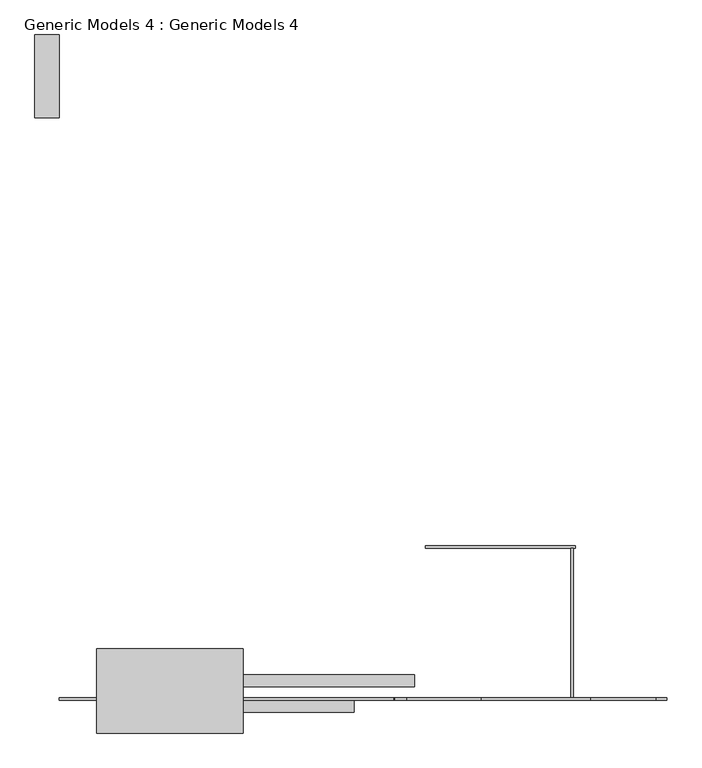
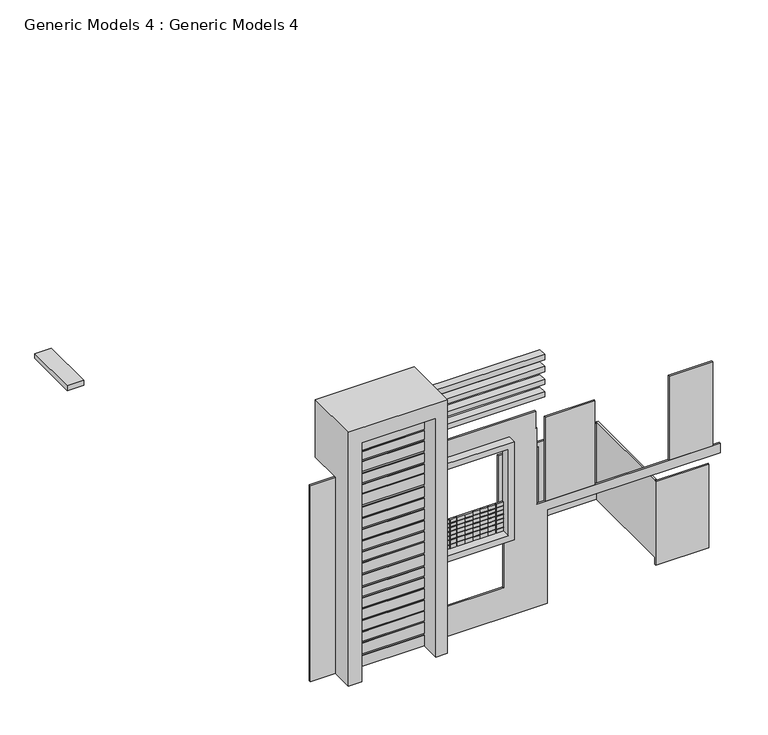
"""IFC4 building model written with IfcOpenShell, lengths in millimetres: proxy geometry, Generic Models 4 : Generic Models 4."""

from ifc_helpers import new_model, si_unit, frame, origin, origin_with_axes, place, context, project, spatial, polyline, outline, extrude, faceted_brep, source, transform, mapped, element, save


def generic_models_4_generic_models_4_67bf9aa9(model_context):
    return source(origin(), model_context, "Body", "SolidModel", [
        extrude(outline(polyline([(-19874.3127664, -11976.0511954), (-19874.3127664, -11725.3336873), (-16074.1386697, -11725.3336873), (-16074.1386697, -11976.0511954), (-19874.3127664, -11976.0511954)])), frame((0.0, 0.0, 7756.9299202), z_axis=(0.0, 0.0, 1.0), x_axis=(1.0, 0.0, 0.0)), (0.0, 0.0, 1.0), 173.7908579),
        extrude(outline(polyline([(-19874.3127664, -11976.0511954), (-19874.3127664, -11725.3336873), (-16074.1386697, -11725.3336873), (-16074.1386697, -11976.0511954), (-19874.3127664, -11976.0511954)])), frame((0.0, 0.0, 7363.4945903), z_axis=(0.0, 0.0, 1.0), x_axis=(1.0, 0.0, 0.0)), (0.0, 0.0, 1.0), 172.4010314),
        extrude(outline(polyline([(-19874.3127664, -11976.0511954), (-19874.3127664, -11725.3336873), (-16074.1386697, -11725.3336873), (-16074.1386697, -11976.0511954), (-19874.3127664, -11976.0511954)])), frame((0.0, 0.0, 6958.2524278), z_axis=(0.0, 0.0, 1.0), x_axis=(1.0, 0.0, 0.0)), (0.0, 0.0, 1.0), 155.6173334),
        extrude(outline(polyline([(-19874.3127664, -11976.0511954), (-19874.3127664, -11725.3336873), (-16074.1386697, -11725.3336873), (-16074.1386697, -11976.0511954), (-19874.3127664, -11976.0511954)])), frame((0.0, 0.0, 6536.8664584), z_axis=(0.0, 0.0, 1.0), x_axis=(1.0, 0.0, 0.0)), (0.0, 0.0, 1.0), 161.3441341),
        extrude(outline(polyline([(-23975.6647706, 1587.5488046), (-23465.5386697, 1587.5488046), (-23465.5386697, -136.4761954), (-23975.6647706, -136.4761954), (-23975.6647706, 1587.5488046)])), frame((0.0, 0.0, 2332.8596388), z_axis=(0.0, 0.0, 1.0), x_axis=(1.0, 0.0, 0.0)), (0.0, 0.0, 1.0), 152.4),
        faceted_brep([(-19636.4886697, -12255.4511954, 3784.7260489), (-19636.4886697, -12255.4511954, 3671.2049424), (-19413.4515656, -12255.4511954, 3671.2049424), (-19413.4515656, -12255.4511954, 3784.7260489), (-19636.4886697, -12255.4511954, 3649.7991228), (-19636.4886697, -12255.4511954, 3542.7700248), (-19413.4515656, -12255.4511954, 3542.7700248), (-19413.4515656, -12255.4511954, 3649.7991228), (-19636.4886697, -12255.4511954, 3518.306231), (-19636.4886697, -12255.4511954, 3408.2191587), (-19413.4515656, -12255.4511954, 3408.2191587), (-19413.4515656, -12255.4511954, 3518.306231), (-19636.4886697, -12255.4511954, 3383.7553649), (-19636.4886697, -12255.4511954, 3271.5066224), (-19413.4515656, -12255.4511954, 3271.5066224), (-19413.4515656, -12255.4511954, 3383.7553649), (-19636.4886697, -12255.4511954, 3255.3204473), (-19636.4886697, -12255.4511954, 3137.364874), (-19413.4515656, -12255.4511954, 3137.364874), (-19413.4515656, -12255.4511954, 3255.3204473), (-19636.4886697, -12255.4511954, 2960.0023687), (-19636.4886697, -12255.4511954, 2833.3789545), (-19413.4515656, -12255.4511954, 2833.3789545), (-19413.4515656, -12255.4511954, 2960.0023687), (-19636.4886697, -12255.4511954, 3112.9010801), (-19636.4886697, -12255.4511954, 2978.3502141), (-19413.4515656, -12255.4511954, 2978.3502141), (-19413.4515656, -12255.4511954, 3112.9010801), (-17502.8886697, -12255.4511954, 3671.2049424), (-17502.8886697, -12255.4511954, 3784.7260489), (-17737.0072187, -12255.4511954, 3784.7260489), (-17737.0072187, -12255.4511954, 3671.2049424), (-17502.8886697, -12255.4511954, 3542.7700248), (-17502.8886697, -12255.4511954, 3649.7991228), (-17737.0072187, -12255.4511954, 3649.7991228), (-17737.0072187, -12255.4511954, 3542.7700248), (-17502.8886697, -12255.4511954, 3408.2191587), (-17502.8886697, -12255.4511954, 3518.306231), (-17737.0072187, -12255.4511954, 3518.306231), (-17737.0072187, -12255.4511954, 3408.2191587), (-17502.8886697, -12255.4511954, 3271.5066224), (-17502.8886697, -12255.4511954, 3383.7553649), (-17737.0072187, -12255.4511954, 3383.7553649), (-17737.0072187, -12255.4511954, 3271.5066224), (-17502.8886697, -12255.4511954, 3137.364874), (-17502.8886697, -12255.4511954, 3255.3204473), (-17737.0072187, -12255.4511954, 3255.3204473), (-17737.0072187, -12255.4511954, 3137.364874), (-17502.8886697, -12255.4511954, 2833.3789545), (-17502.8886697, -12255.4511954, 2960.0023687), (-17737.0072187, -12255.4511954, 2960.0023687), (-17737.0072187, -12255.4511954, 2833.3789545), (-17502.8886697, -12255.4511954, 2978.3502141), (-17502.8886697, -12255.4511954, 3112.9010801), (-17737.0072187, -12255.4511954, 3112.9010801), (-17737.0072187, -12255.4511954, 2978.3502141), (-19182.4143994, -12255.4511954, 3784.7260489), (-19387.1657173, -12255.4511954, 3784.7260489), (-19387.1657173, -12255.4511954, 3671.2049424), (-19182.4143994, -12255.4511954, 3671.2049424), (-18957.0386697, -12255.4511954, 3784.7260489), (-19153.1642111, -12255.4511954, 3784.7260489), (-19153.1642111, -12255.4511954, 3671.2049424), (-18957.0386697, -12255.4511954, 3671.2049424), (-18703.0386697, -12255.4511954, 3784.7260489), (-18927.140029, -12255.4511954, 3784.7260489), (-18927.140029, -12255.4511954, 3671.2049424), (-18703.0386697, -12255.4511954, 3671.2049424), (-18461.2038197, -12255.4511954, 3784.7260489), (-18685.5210952, -12255.4511954, 3784.7260489), (-18685.5210952, -12255.4511954, 3671.2049424), (-18461.2038197, -12255.4511954, 3671.2049424), (-18245.8386697, -12255.4511954, 3784.7260489), (-18433.5803118, -12255.4511954, 3784.7260489), (-18433.5803118, -12255.4511954, 3671.2049424), (-18245.8386697, -12255.4511954, 3671.2049424), (-17998.1886697, -12255.4511954, 3784.7260489), (-18218.7706288, -12255.4511954, 3784.7260489), (-18218.7706288, -12255.4511954, 3671.2049424), (-17998.1886697, -12255.4511954, 3671.2049424), (-17756.5762606, -12255.4511954, 3784.7260489), (-17975.8395726, -12255.4511954, 3784.7260489), (-17975.8395726, -12255.4511954, 3671.2049424), (-17756.5762606, -12255.4511954, 3671.2049424), (-19387.1657173, -12255.4511954, 2833.3789545), (-19182.4143994, -12255.4511954, 2833.3789545), (-19182.4143994, -12255.4511954, 2960.0023687), (-19387.1657173, -12255.4511954, 2960.0023687), (-19153.1642111, -12255.4511954, 2833.3789545), (-18957.0386697, -12255.4511954, 2833.3789545), (-18957.0386697, -12255.4511954, 2960.0023687), (-19153.1642111, -12255.4511954, 2960.0023687), (-18927.140029, -12255.4511954, 2833.3789545), (-18703.0386697, -12255.4511954, 2833.3789545), (-18703.0386697, -12255.4511954, 2960.0023687), (-18927.140029, -12255.4511954, 2960.0023687), (-18685.5210952, -12255.4511954, 2833.3789545), (-18461.2038197, -12255.4511954, 2833.3789545), (-18461.2038197, -12255.4511954, 2960.0023687), (-18685.5210952, -12255.4511954, 2960.0023687), (-18433.5803118, -12255.4511954, 2833.3789545), (-18245.8386697, -12255.4511954, 2833.3789545), (-18245.8386697, -12255.4511954, 2960.0023687), (-18433.5803118, -12255.4511954, 2960.0023687), (-18218.7706288, -12255.4511954, 2833.3789545), (-17998.1886697, -12255.4511954, 2833.3789545), (-17998.1886697, -12255.4511954, 2960.0023687), (-18218.7706288, -12255.4511954, 2960.0023687), (-17975.8395726, -12255.4511954, 2833.3789545), (-17756.5762606, -12255.4511954, 2833.3789545), (-17756.5762606, -12255.4511954, 2960.0023687), (-17975.8395726, -12255.4511954, 2960.0023687), (-19387.1657173, -12255.4511954, 3542.7700248), (-19182.4143994, -12255.4511954, 3542.7700248), (-19182.4143994, -12255.4511954, 3649.7991228), (-19387.1657173, -12255.4511954, 3649.7991228), (-19153.1642111, -12255.4511954, 3542.7700248), (-18957.0386697, -12255.4511954, 3542.7700248), (-18957.0386697, -12255.4511954, 3649.7991228), (-19153.1642111, -12255.4511954, 3649.7991228), (-18927.140029, -12255.4511954, 3542.7700248), (-18703.0386697, -12255.4511954, 3542.7700248), (-18703.0386697, -12255.4511954, 3649.7991228), (-18927.140029, -12255.4511954, 3649.7991228), (-18685.5210952, -12255.4511954, 3542.7700248), (-18461.2038197, -12255.4511954, 3542.7700248), (-18461.2038197, -12255.4511954, 3649.7991228), (-18685.5210952, -12255.4511954, 3649.7991228), (-18433.5803118, -12255.4511954, 3542.7700248), (-18245.8386697, -12255.4511954, 3542.7700248), (-18245.8386697, -12255.4511954, 3649.7991228), (-18433.5803118, -12255.4511954, 3649.7991228), (-18218.7706288, -12255.4511954, 3542.7700248), (-17998.1886697, -12255.4511954, 3542.7700248), (-17998.1886697, -12255.4511954, 3649.7991228), (-18218.7706288, -12255.4511954, 3649.7991228), (-17975.8395726, -12255.4511954, 3542.7700248), (-17756.5762606, -12255.4511954, 3542.7700248), (-17756.5762606, -12255.4511954, 3649.7991228), (-17975.8395726, -12255.4511954, 3649.7991228), (-19387.1657173, -12255.4511954, 3408.2191587), (-19182.4143994, -12255.4511954, 3408.2191587), (-19182.4143994, -12255.4511954, 3518.306231), (-19387.1657173, -12255.4511954, 3518.306231), (-19153.1642111, -12255.4511954, 3408.2191587), (-18957.0386697, -12255.4511954, 3408.2191587), (-18957.0386697, -12255.4511954, 3518.306231), (-19153.1642111, -12255.4511954, 3518.306231), (-18927.140029, -12255.4511954, 3408.2191587), (-18703.0386697, -12255.4511954, 3408.2191587), (-18703.0386697, -12255.4511954, 3518.306231), (-18927.140029, -12255.4511954, 3518.306231), (-18685.5210952, -12255.4511954, 3408.2191587), (-18461.2038197, -12255.4511954, 3408.2191587), (-18461.2038197, -12255.4511954, 3518.306231), (-18685.5210952, -12255.4511954, 3518.306231), (-18433.5803118, -12255.4511954, 3408.2191587), (-18245.8386697, -12255.4511954, 3408.2191587), (-18245.8386697, -12255.4511954, 3518.306231), (-18433.5803118, -12255.4511954, 3518.306231), (-18218.7706288, -12255.4511954, 3408.2191587), (-17998.1886697, -12255.4511954, 3408.2191587), (-17998.1886697, -12255.4511954, 3518.306231), (-18218.7706288, -12255.4511954, 3518.306231), (-17975.8395726, -12255.4511954, 3408.2191587), (-17756.5762606, -12255.4511954, 3408.2191587), (-17756.5762606, -12255.4511954, 3518.306231), (-17975.8395726, -12255.4511954, 3518.306231), (-19387.1657173, -12255.4511954, 3271.5066224), (-19182.4143994, -12255.4511954, 3271.5066224), (-19182.4143994, -12255.4511954, 3383.7553649), (-19387.1657173, -12255.4511954, 3383.7553649), (-19153.1642111, -12255.4511954, 3271.5066224), (-18957.0386697, -12255.4511954, 3271.5066224), (-18957.0386697, -12255.4511954, 3383.7553649), (-19153.1642111, -12255.4511954, 3383.7553649), (-18927.140029, -12255.4511954, 3271.5066224), (-18703.0386697, -12255.4511954, 3271.5066224), (-18703.0386697, -12255.4511954, 3383.7553649), (-18927.140029, -12255.4511954, 3383.7553649), (-18685.5210952, -12255.4511954, 3271.5066224), (-18461.2038197, -12255.4511954, 3271.5066224), (-18461.2038197, -12255.4511954, 3383.7553649), (-18685.5210952, -12255.4511954, 3383.7553649), (-18433.5803118, -12255.4511954, 3271.5066224), (-18245.8386697, -12255.4511954, 3271.5066224), (-18245.8386697, -12255.4511954, 3383.7553649), (-18433.5803118, -12255.4511954, 3383.7553649), (-18218.7706288, -12255.4511954, 3271.5066224), (-17998.1886697, -12255.4511954, 3271.5066224), (-17998.1886697, -12255.4511954, 3383.7553649), (-18218.7706288, -12255.4511954, 3383.7553649), (-17975.8395726, -12255.4511954, 3271.5066224), (-17756.5762606, -12255.4511954, 3271.5066224), (-17756.5762606, -12255.4511954, 3383.7553649), (-17975.8395726, -12255.4511954, 3383.7553649), (-19387.1657173, -12255.4511954, 3137.364874), (-19182.4143994, -12255.4511954, 3137.364874), (-19182.4143994, -12255.4511954, 3255.3204473), (-19387.1657173, -12255.4511954, 3255.3204473), (-19153.1642111, -12255.4511954, 3137.364874), (-18957.0386697, -12255.4511954, 3137.364874), (-18957.0386697, -12255.4511954, 3255.3204473), (-19153.1642111, -12255.4511954, 3255.3204473), (-18927.140029, -12255.4511954, 3137.364874), (-18703.0386697, -12255.4511954, 3137.364874), (-18703.0386697, -12255.4511954, 3255.3204473), (-18927.140029, -12255.4511954, 3255.3204473), (-18685.5210952, -12255.4511954, 3137.364874), (-18461.2038197, -12255.4511954, 3137.364874), (-18461.2038197, -12255.4511954, 3255.3204473), (-18685.5210952, -12255.4511954, 3255.3204473), (-18433.5803118, -12255.4511954, 3137.364874), (-18245.8386697, -12255.4511954, 3137.364874), (-18245.8386697, -12255.4511954, 3255.3204473), (-18433.5803118, -12255.4511954, 3255.3204473), (-18218.7706288, -12255.4511954, 3137.364874), (-17998.1886697, -12255.4511954, 3137.364874), (-17998.1886697, -12255.4511954, 3255.3204473), (-18218.7706288, -12255.4511954, 3255.3204473), (-17975.8395726, -12255.4511954, 3137.364874), (-17756.5762606, -12255.4511954, 3137.364874), (-17756.5762606, -12255.4511954, 3255.3204473), (-17975.8395726, -12255.4511954, 3255.3204473), (-19387.1657173, -12255.4511954, 2978.3502141), (-19182.4143994, -12255.4511954, 2978.3502141), (-19182.4143994, -12255.4511954, 3112.9010801), (-19387.1657173, -12255.4511954, 3112.9010801), (-19153.1642111, -12255.4511954, 2978.3502141), (-18957.0386697, -12255.4511954, 2978.3502141), (-18957.0386697, -12255.4511954, 3112.9010801), (-19153.1642111, -12255.4511954, 3112.9010801), (-18927.140029, -12255.4511954, 2978.3502141), (-18703.0386697, -12255.4511954, 2978.3502141), (-18703.0386697, -12255.4511954, 3112.9010801), (-18927.140029, -12255.4511954, 3112.9010801), (-18685.5210952, -12255.4511954, 2978.3502141), (-18461.2038197, -12255.4511954, 2978.3502141), (-18461.2038197, -12255.4511954, 3112.9010801), (-18685.5210952, -12255.4511954, 3112.9010801), (-18433.5803118, -12255.4511954, 2978.3502141), (-18245.8386697, -12255.4511954, 2978.3502141), (-18245.8386697, -12255.4511954, 3112.9010801), (-18433.5803118, -12255.4511954, 3112.9010801), (-18218.7706288, -12255.4511954, 2978.3502141), (-17998.1886697, -12255.4511954, 2978.3502141), (-17998.1886697, -12255.4511954, 3112.9010801), (-18218.7706288, -12255.4511954, 3112.9010801), (-17975.8395726, -12255.4511954, 2978.3502141), (-17756.5762606, -12255.4511954, 2978.3502141), (-17756.5762606, -12255.4511954, 3112.9010801), (-17975.8395726, -12255.4511954, 3112.9010801), (-17502.8886697, -12204.6511954, 3784.7260489), (-17502.8886697, -12204.6511954, 2833.3789545), (-19636.4886697, -12204.6511954, 2833.3789545), (-19636.4886697, -12204.6511954, 3784.7260489), (-19413.4515656, -12230.0511954, 3784.7260489), (-19387.1657173, -12230.0511954, 3784.7260489), (-19182.4143994, -12230.0511954, 3784.7260489), (-19153.1642111, -12230.0511954, 3784.7260489), (-18957.0386697, -12230.0511954, 3784.7260489), (-18927.140029, -12230.0511954, 3784.7260489), (-18703.0386697, -12230.0511954, 3784.7260489), (-18685.5210952, -12230.0511954, 3784.7260489), (-18461.2038197, -12230.0511954, 3784.7260489), (-18433.5803118, -12230.0511954, 3784.7260489), (-18245.8386697, -12230.0511954, 3784.7260489), (-18218.7706288, -12230.0511954, 3784.7260489), (-17998.1886697, -12230.0511954, 3784.7260489), (-17975.8395726, -12230.0511954, 3784.7260489), (-17756.5762606, -12230.0511954, 3784.7260489), (-17737.0072187, -12230.0511954, 3784.7260489), (-19636.4886697, -12230.0511954, 2960.0023687), (-19636.4886697, -12230.0511954, 2978.3502141), (-19636.4886697, -12230.0511954, 3112.9010801), (-19636.4886697, -12230.0511954, 3137.364874), (-19636.4886697, -12230.0511954, 3255.3204473), (-19636.4886697, -12230.0511954, 3271.5066224), (-19636.4886697, -12230.0511954, 3383.7553649), (-19636.4886697, -12230.0511954, 3408.2191587), (-19636.4886697, -12230.0511954, 3518.306231), (-19636.4886697, -12230.0511954, 3542.7700248), (-19636.4886697, -12230.0511954, 3649.7991228), (-19636.4886697, -12230.0511954, 3671.2049424), (-17737.0072187, -12230.0511954, 2833.3789545), (-17756.5762606, -12230.0511954, 2833.3789545), (-17975.8395726, -12230.0511954, 2833.3789545), (-17998.1886697, -12230.0511954, 2833.3789545), (-18218.7706288, -12230.0511954, 2833.3789545), (-18245.8386697, -12230.0511954, 2833.3789545), (-18433.5803118, -12230.0511954, 2833.3789545), (-18461.2038197, -12230.0511954, 2833.3789545), (-18685.5210952, -12230.0511954, 2833.3789545), (-18703.0386697, -12230.0511954, 2833.3789545), (-18927.140029, -12230.0511954, 2833.3789545), (-18957.0386697, -12230.0511954, 2833.3789545), (-19153.1642111, -12230.0511954, 2833.3789545), (-19182.4143994, -12230.0511954, 2833.3789545), (-19387.1657173, -12230.0511954, 2833.3789545), (-19413.4515656, -12230.0511954, 2833.3789545), (-17502.8886697, -12230.0511954, 3671.2049424), (-17502.8886697, -12230.0511954, 3649.7991228), (-17502.8886697, -12230.0511954, 3542.7700248), (-17502.8886697, -12230.0511954, 3518.306231), (-17502.8886697, -12230.0511954, 3408.2191587), (-17502.8886697, -12230.0511954, 3383.7553649), (-17502.8886697, -12230.0511954, 3271.5066224), (-17502.8886697, -12230.0511954, 3255.3204473), (-17502.8886697, -12230.0511954, 3137.364874), (-17502.8886697, -12230.0511954, 3112.9010801), (-17502.8886697, -12230.0511954, 2978.3502141), (-17502.8886697, -12230.0511954, 2960.0023687), (-19413.4515656, -12230.0511954, 3649.7991228), (-19413.4515656, -12230.0511954, 3542.7700248), (-19413.4515656, -12230.0511954, 3518.306231), (-19413.4515656, -12230.0511954, 3408.2191587), (-19413.4515656, -12230.0511954, 3383.7553649), (-19413.4515656, -12230.0511954, 3271.5066224), (-19413.4515656, -12230.0511954, 3255.3204473), (-19413.4515656, -12230.0511954, 3137.364874), (-19413.4515656, -12230.0511954, 3112.9010801), (-19413.4515656, -12230.0511954, 2978.3502141), (-19413.4515656, -12230.0511954, 2960.0023687), (-19387.1657173, -12230.0511954, 2960.0023687), (-19182.4143994, -12230.0511954, 2960.0023687), (-19153.1642111, -12230.0511954, 2960.0023687), (-18957.0386697, -12230.0511954, 2960.0023687), (-18927.140029, -12230.0511954, 2960.0023687), (-18703.0386697, -12230.0511954, 2960.0023687), (-18685.5210952, -12230.0511954, 2960.0023687), (-18461.2038197, -12230.0511954, 2960.0023687), (-18433.5803118, -12230.0511954, 2960.0023687), (-18245.8386697, -12230.0511954, 2960.0023687), (-18218.7706288, -12230.0511954, 2960.0023687), (-17998.1886697, -12230.0511954, 2960.0023687), (-17975.8395726, -12230.0511954, 2960.0023687), (-17756.5762606, -12230.0511954, 2960.0023687), (-17737.0072187, -12230.0511954, 2960.0023687), (-17737.0072187, -12230.0511954, 2978.3502141), (-17737.0072187, -12230.0511954, 3112.9010801), (-17737.0072187, -12230.0511954, 3137.364874), (-17737.0072187, -12230.0511954, 3255.3204473), (-17737.0072187, -12230.0511954, 3271.5066224), (-17737.0072187, -12230.0511954, 3383.7553649), (-17737.0072187, -12230.0511954, 3408.2191587), (-17737.0072187, -12230.0511954, 3518.306231), (-17737.0072187, -12230.0511954, 3542.7700248), (-17737.0072187, -12230.0511954, 3649.7991228), (-17737.0072187, -12230.0511954, 3671.2049424), (-17756.5762606, -12230.0511954, 3671.2049424), (-17975.8395726, -12230.0511954, 3671.2049424), (-17998.1886697, -12230.0511954, 3671.2049424), (-18218.7706288, -12230.0511954, 3671.2049424), (-18245.8386697, -12230.0511954, 3671.2049424), (-18433.5803118, -12230.0511954, 3671.2049424), (-18461.2038197, -12230.0511954, 3671.2049424), (-18685.5210952, -12230.0511954, 3671.2049424), (-18703.0386697, -12230.0511954, 3671.2049424), (-18927.140029, -12230.0511954, 3671.2049424), (-18957.0386697, -12230.0511954, 3671.2049424), (-19153.1642111, -12230.0511954, 3671.2049424), (-19182.4143994, -12230.0511954, 3671.2049424), (-19387.1657173, -12230.0511954, 3671.2049424), (-19413.4515656, -12230.0511954, 3671.2049424), (-19387.1657173, -12230.0511954, 3649.7991228), (-19182.4143994, -12230.0511954, 3649.7991228), (-19182.4143994, -12230.0511954, 3542.7700248), (-19387.1657173, -12230.0511954, 3542.7700248), (-19153.1642111, -12230.0511954, 3649.7991228), (-18957.0386697, -12230.0511954, 3649.7991228), (-18957.0386697, -12230.0511954, 3542.7700248), (-19153.1642111, -12230.0511954, 3542.7700248), (-18927.140029, -12230.0511954, 3649.7991228), (-18703.0386697, -12230.0511954, 3649.7991228), (-18703.0386697, -12230.0511954, 3542.7700248), (-18927.140029, -12230.0511954, 3542.7700248), (-18685.5210952, -12230.0511954, 3649.7991228), (-18461.2038197, -12230.0511954, 3649.7991228), (-18461.2038197, -12230.0511954, 3542.7700248), (-18685.5210952, -12230.0511954, 3542.7700248), (-18433.5803118, -12230.0511954, 3649.7991228), (-18245.8386697, -12230.0511954, 3649.7991228), (-18245.8386697, -12230.0511954, 3542.7700248), (-18433.5803118, -12230.0511954, 3542.7700248), (-18218.7706288, -12230.0511954, 3649.7991228), (-17998.1886697, -12230.0511954, 3649.7991228), (-17998.1886697, -12230.0511954, 3542.7700248), (-18218.7706288, -12230.0511954, 3542.7700248), (-17975.8395726, -12230.0511954, 3649.7991228), (-17756.5762606, -12230.0511954, 3649.7991228), (-17756.5762606, -12230.0511954, 3542.7700248), (-17975.8395726, -12230.0511954, 3542.7700248), (-19387.1657173, -12230.0511954, 3518.306231), (-19182.4143994, -12230.0511954, 3518.306231), (-19182.4143994, -12230.0511954, 3408.2191587), (-19387.1657173, -12230.0511954, 3408.2191587), (-19153.1642111, -12230.0511954, 3518.306231), (-18957.0386697, -12230.0511954, 3518.306231), (-18957.0386697, -12230.0511954, 3408.2191587), (-19153.1642111, -12230.0511954, 3408.2191587), (-18927.140029, -12230.0511954, 3518.306231), (-18703.0386697, -12230.0511954, 3518.306231), (-18703.0386697, -12230.0511954, 3408.2191587), (-18927.140029, -12230.0511954, 3408.2191587), (-18685.5210952, -12230.0511954, 3518.306231), (-18461.2038197, -12230.0511954, 3518.306231), (-18461.2038197, -12230.0511954, 3408.2191587), (-18685.5210952, -12230.0511954, 3408.2191587), (-18433.5803118, -12230.0511954, 3518.306231), (-18245.8386697, -12230.0511954, 3518.306231), (-18245.8386697, -12230.0511954, 3408.2191587), (-18433.5803118, -12230.0511954, 3408.2191587), (-18218.7706288, -12230.0511954, 3518.306231), (-17998.1886697, -12230.0511954, 3518.306231), (-17998.1886697, -12230.0511954, 3408.2191587), (-18218.7706288, -12230.0511954, 3408.2191587), (-17975.8395726, -12230.0511954, 3518.306231), (-17756.5762606, -12230.0511954, 3518.306231), (-17756.5762606, -12230.0511954, 3408.2191587), (-17975.8395726, -12230.0511954, 3408.2191587), (-19387.1657173, -12230.0511954, 3383.7553649), (-19182.4143994, -12230.0511954, 3383.7553649), (-19182.4143994, -12230.0511954, 3271.5066224), (-19387.1657173, -12230.0511954, 3271.5066224), (-19153.1642111, -12230.0511954, 3383.7553649), (-18957.0386697, -12230.0511954, 3383.7553649), (-18957.0386697, -12230.0511954, 3271.5066224), (-19153.1642111, -12230.0511954, 3271.5066224), (-18927.140029, -12230.0511954, 3383.7553649), (-18703.0386697, -12230.0511954, 3383.7553649), (-18703.0386697, -12230.0511954, 3271.5066224), (-18927.140029, -12230.0511954, 3271.5066224), (-18685.5210952, -12230.0511954, 3383.7553649), (-18461.2038197, -12230.0511954, 3383.7553649), (-18461.2038197, -12230.0511954, 3271.5066224), (-18685.5210952, -12230.0511954, 3271.5066224), (-18433.5803118, -12230.0511954, 3383.7553649), (-18245.8386697, -12230.0511954, 3383.7553649), (-18245.8386697, -12230.0511954, 3271.5066224), (-18433.5803118, -12230.0511954, 3271.5066224), (-18218.7706288, -12230.0511954, 3383.7553649), (-17998.1886697, -12230.0511954, 3383.7553649), (-17998.1886697, -12230.0511954, 3271.5066224), (-18218.7706288, -12230.0511954, 3271.5066224), (-17975.8395726, -12230.0511954, 3383.7553649), (-17756.5762606, -12230.0511954, 3383.7553649), (-17756.5762606, -12230.0511954, 3271.5066224), (-17975.8395726, -12230.0511954, 3271.5066224), (-19387.1657173, -12230.0511954, 3255.3204473), (-19182.4143994, -12230.0511954, 3255.3204473), (-19182.4143994, -12230.0511954, 3137.364874), (-19387.1657173, -12230.0511954, 3137.364874), (-19153.1642111, -12230.0511954, 3255.3204473), (-18957.0386697, -12230.0511954, 3255.3204473), (-18957.0386697, -12230.0511954, 3137.364874), (-19153.1642111, -12230.0511954, 3137.364874), (-18927.140029, -12230.0511954, 3255.3204473), (-18703.0386697, -12230.0511954, 3255.3204473), (-18703.0386697, -12230.0511954, 3137.364874), (-18927.140029, -12230.0511954, 3137.364874), (-18685.5210952, -12230.0511954, 3255.3204473), (-18461.2038197, -12230.0511954, 3255.3204473), (-18461.2038197, -12230.0511954, 3137.364874), (-18685.5210952, -12230.0511954, 3137.364874), (-18433.5803118, -12230.0511954, 3255.3204473), (-18245.8386697, -12230.0511954, 3255.3204473), (-18245.8386697, -12230.0511954, 3137.364874), (-18433.5803118, -12230.0511954, 3137.364874), (-18218.7706288, -12230.0511954, 3255.3204473), (-17998.1886697, -12230.0511954, 3255.3204473), (-17998.1886697, -12230.0511954, 3137.364874), (-18218.7706288, -12230.0511954, 3137.364874), (-17975.8395726, -12230.0511954, 3255.3204473), (-17756.5762606, -12230.0511954, 3255.3204473), (-17756.5762606, -12230.0511954, 3137.364874), (-17975.8395726, -12230.0511954, 3137.364874), (-19387.1657173, -12230.0511954, 3112.9010801), (-19182.4143994, -12230.0511954, 3112.9010801), (-19182.4143994, -12230.0511954, 2978.3502141), (-19387.1657173, -12230.0511954, 2978.3502141), (-19153.1642111, -12230.0511954, 3112.9010801), (-18957.0386697, -12230.0511954, 3112.9010801), (-18957.0386697, -12230.0511954, 2978.3502141), (-19153.1642111, -12230.0511954, 2978.3502141), (-18927.140029, -12230.0511954, 3112.9010801), (-18703.0386697, -12230.0511954, 3112.9010801), (-18703.0386697, -12230.0511954, 2978.3502141), (-18927.140029, -12230.0511954, 2978.3502141), (-18685.5210952, -12230.0511954, 3112.9010801), (-18461.2038197, -12230.0511954, 3112.9010801), (-18461.2038197, -12230.0511954, 2978.3502141), (-18685.5210952, -12230.0511954, 2978.3502141), (-18433.5803118, -12230.0511954, 3112.9010801), (-18245.8386697, -12230.0511954, 3112.9010801), (-18245.8386697, -12230.0511954, 2978.3502141), (-18433.5803118, -12230.0511954, 2978.3502141), (-18218.7706288, -12230.0511954, 3112.9010801), (-17998.1886697, -12230.0511954, 3112.9010801), (-17998.1886697, -12230.0511954, 2978.3502141), (-18218.7706288, -12230.0511954, 2978.3502141), (-17975.8395726, -12230.0511954, 3112.9010801), (-17756.5762606, -12230.0511954, 3112.9010801), (-17756.5762606, -12230.0511954, 2978.3502141), (-17975.8395726, -12230.0511954, 2978.3502141)], [[[0, 1, 2, 3]], [[4, 5, 6, 7]], [[8, 9, 10, 11]], [[12, 13, 14, 15]], [[16, 17, 18, 19]], [[20, 21, 22, 23]], [[24, 25, 26, 27]], [[28, 29, 30, 31]], [[32, 33, 34, 35]], [[36, 37, 38, 39]], [[40, 41, 42, 43]], [[44, 45, 46, 47]], [[48, 49, 50, 51]], [[52, 53, 54, 55]], [[56, 57, 58, 59]], [[60, 61, 62, 63]], [[64, 65, 66, 67]], [[68, 69, 70, 71]], [[72, 73, 74, 75]], [[76, 77, 78, 79]], [[80, 81, 82, 83]], [[84, 85, 86, 87]], [[88, 89, 90, 91]], [[92, 93, 94, 95]], [[96, 97, 98, 99]], [[100, 101, 102, 103]], [[104, 105, 106, 107]], [[108, 109, 110, 111]], [[112, 113, 114, 115]], [[116, 117, 118, 119]], [[120, 121, 122, 123]], [[124, 125, 126, 127]], [[128, 129, 130, 131]], [[132, 133, 134, 135]], [[136, 137, 138, 139]], [[140, 141, 142, 143]], [[144, 145, 146, 147]], [[148, 149, 150, 151]], [[152, 153, 154, 155]], [[156, 157, 158, 159]], [[160, 161, 162, 163]], [[164, 165, 166, 167]], [[168, 169, 170, 171]], [[172, 173, 174, 175]], [[176, 177, 178, 179]], [[180, 181, 182, 183]], [[184, 185, 186, 187]], [[188, 189, 190, 191]], [[192, 193, 194, 195]], [[196, 197, 198, 199]], [[200, 201, 202, 203]], [[204, 205, 206, 207]], [[208, 209, 210, 211]], [[212, 213, 214, 215]], [[216, 217, 218, 219]], [[220, 221, 222, 223]], [[224, 225, 226, 227]], [[228, 229, 230, 231]], [[232, 233, 234, 235]], [[236, 237, 238, 239]], [[240, 241, 242, 243]], [[244, 245, 246, 247]], [[248, 249, 250, 251]], [[252, 253, 254, 255]], [[252, 255, 0, 3, 256, 257, 57, 56, 258, 259, 61, 60, 260, 261, 65, 64, 262, 263, 69, 68, 264, 265, 73, 72, 266, 267, 77, 76, 268, 269, 81, 80, 270, 271, 30, 29]], [[255, 254, 21, 20, 272, 273, 25, 24, 274, 275, 17, 16, 276, 277, 13, 12, 278, 279, 9, 8, 280, 281, 5, 4, 282, 283, 1, 0]], [[254, 253, 48, 51, 284, 285, 109, 108, 286, 287, 105, 104, 288, 289, 101, 100, 290, 291, 97, 96, 292, 293, 93, 92, 294, 295, 89, 88, 296, 297, 85, 84, 298, 299, 22, 21]], [[253, 252, 29, 28, 300, 301, 33, 32, 302, 303, 37, 36, 304, 305, 41, 40, 306, 307, 45, 44, 308, 309, 53, 52, 310, 311, 49, 48]], [[283, 282, 312, 313, 281, 280, 314, 315, 279, 278, 316, 317, 277, 276, 318, 319, 275, 274, 320, 321, 273, 272, 322, 299, 298, 323, 324, 297, 296, 325, 326, 295, 294, 327, 328, 293, 292, 329, 330, 291, 290, 331, 332, 289, 288, 333, 334, 287, 286, 335, 336, 285, 284, 337, 311, 310, 338, 339, 309, 308, 340, 341, 307, 306, 342, 343, 305, 304, 344, 345, 303, 302, 346, 347, 301, 300, 348, 271, 270, 349, 350, 269, 268, 351, 352, 267, 266, 353, 354, 265, 264, 355, 356, 263, 262, 357, 358, 261, 260, 359, 360, 259, 258, 361, 362, 257, 256, 363], [364, 365, 366, 367], [368, 369, 370, 371], [372, 373, 374, 375], [376, 377, 378, 379], [380, 381, 382, 383], [384, 385, 386, 387], [388, 389, 390, 391], [392, 393, 394, 395], [396, 397, 398, 399], [400, 401, 402, 403], [404, 405, 406, 407], [408, 409, 410, 411], [412, 413, 414, 415], [416, 417, 418, 419], [420, 421, 422, 423], [424, 425, 426, 427], [428, 429, 430, 431], [432, 433, 434, 435], [436, 437, 438, 439], [440, 441, 442, 443], [444, 445, 446, 447], [448, 449, 450, 451], [452, 453, 454, 455], [456, 457, 458, 459], [460, 461, 462, 463], [464, 465, 466, 467], [468, 469, 470, 471], [472, 473, 474, 475], [476, 477, 478, 479], [480, 481, 482, 483], [484, 485, 486, 487], [488, 489, 490, 491], [492, 493, 494, 495], [496, 497, 498, 499], [500, 501, 502, 503]], [[115, 114, 365, 364]], [[119, 118, 369, 368]], [[123, 122, 373, 372]], [[127, 126, 377, 376]], [[131, 130, 381, 380]], [[135, 134, 385, 384]], [[139, 138, 389, 388]], [[282, 4, 7, 312]], [[33, 301, 347, 34]], [[59, 58, 362, 361]], [[63, 62, 360, 359]], [[67, 66, 358, 357]], [[71, 70, 356, 355]], [[75, 74, 354, 353]], [[79, 78, 352, 351]], [[83, 82, 350, 349]], [[1, 283, 363, 2]], [[300, 28, 31, 348]], [[143, 142, 393, 392]], [[147, 146, 397, 396]], [[151, 150, 401, 400]], [[155, 154, 405, 404]], [[159, 158, 409, 408]], [[163, 162, 413, 412]], [[167, 166, 417, 416]], [[280, 8, 11, 314]], [[37, 303, 345, 38]], [[113, 112, 367, 366]], [[117, 116, 371, 370]], [[121, 120, 375, 374]], [[125, 124, 379, 378]], [[129, 128, 383, 382]], [[133, 132, 387, 386]], [[137, 136, 391, 390]], [[5, 281, 313, 6]], [[302, 32, 35, 346]], [[171, 170, 421, 420]], [[175, 174, 425, 424]], [[179, 178, 429, 428]], [[183, 182, 433, 432]], [[187, 186, 437, 436]], [[191, 190, 441, 440]], [[195, 194, 445, 444]], [[278, 12, 15, 316]], [[41, 305, 343, 42]], [[141, 140, 395, 394]], [[145, 144, 399, 398]], [[149, 148, 403, 402]], [[153, 152, 407, 406]], [[157, 156, 411, 410]], [[161, 160, 415, 414]], [[165, 164, 419, 418]], [[9, 279, 315, 10]], [[304, 36, 39, 344]], [[199, 198, 449, 448]], [[203, 202, 453, 452]], [[207, 206, 457, 456]], [[211, 210, 461, 460]], [[215, 214, 465, 464]], [[219, 218, 469, 468]], [[223, 222, 473, 472]], [[276, 16, 19, 318]], [[45, 307, 341, 46]], [[169, 168, 423, 422]], [[173, 172, 427, 426]], [[177, 176, 431, 430]], [[181, 180, 435, 434]], [[185, 184, 439, 438]], [[189, 188, 443, 442]], [[193, 192, 447, 446]], [[13, 277, 317, 14]], [[306, 40, 43, 342]], [[227, 226, 477, 476]], [[231, 230, 481, 480]], [[235, 234, 485, 484]], [[239, 238, 489, 488]], [[243, 242, 493, 492]], [[247, 246, 497, 496]], [[251, 250, 501, 500]], [[274, 24, 27, 320]], [[53, 309, 339, 54]], [[197, 196, 451, 450]], [[201, 200, 455, 454]], [[205, 204, 459, 458]], [[209, 208, 463, 462]], [[213, 212, 467, 466]], [[217, 216, 471, 470]], [[221, 220, 475, 474]], [[17, 275, 319, 18]], [[308, 44, 47, 340]], [[87, 86, 324, 323]], [[91, 90, 326, 325]], [[95, 94, 328, 327]], [[99, 98, 330, 329]], [[103, 102, 332, 331]], [[107, 106, 334, 333]], [[111, 110, 336, 335]], [[272, 20, 23, 322]], [[49, 311, 337, 50]], [[225, 224, 479, 478]], [[229, 228, 483, 482]], [[233, 232, 487, 486]], [[237, 236, 491, 490]], [[241, 240, 495, 494]], [[245, 244, 499, 498]], [[249, 248, 503, 502]], [[25, 273, 321, 26]], [[310, 52, 55, 338]], [[323, 298, 84, 87]], [[257, 362, 58, 57]], [[364, 367, 112, 115]], [[392, 395, 140, 143]], [[420, 423, 168, 171]], [[448, 451, 196, 199]], [[476, 479, 224, 227]], [[313, 312, 7, 6]], [[315, 314, 11, 10]], [[317, 316, 15, 14]], [[319, 318, 19, 18]], [[321, 320, 27, 26]], [[299, 322, 23, 22]], [[363, 256, 3, 2]], [[325, 296, 88, 91]], [[259, 360, 62, 61]], [[368, 371, 116, 119]], [[396, 399, 144, 147]], [[424, 427, 172, 175]], [[452, 455, 200, 203]], [[480, 483, 228, 231]], [[297, 324, 86, 85]], [[361, 258, 56, 59]], [[366, 365, 114, 113]], [[394, 393, 142, 141]], [[422, 421, 170, 169]], [[450, 449, 198, 197]], [[478, 477, 226, 225]], [[327, 294, 92, 95]], [[261, 358, 66, 65]], [[372, 375, 120, 123]], [[400, 403, 148, 151]], [[428, 431, 176, 179]], [[456, 459, 204, 207]], [[484, 487, 232, 235]], [[295, 326, 90, 89]], [[359, 260, 60, 63]], [[370, 369, 118, 117]], [[398, 397, 146, 145]], [[426, 425, 174, 173]], [[454, 453, 202, 201]], [[482, 481, 230, 229]], [[329, 292, 96, 99]], [[263, 356, 70, 69]], [[376, 379, 124, 127]], [[404, 407, 152, 155]], [[432, 435, 180, 183]], [[460, 463, 208, 211]], [[488, 491, 236, 239]], [[293, 328, 94, 93]], [[357, 262, 64, 67]], [[374, 373, 122, 121]], [[402, 401, 150, 149]], [[430, 429, 178, 177]], [[458, 457, 206, 205]], [[486, 485, 234, 233]], [[331, 290, 100, 103]], [[265, 354, 74, 73]], [[380, 383, 128, 131]], [[408, 411, 156, 159]], [[436, 439, 184, 187]], [[464, 467, 212, 215]], [[492, 495, 240, 243]], [[291, 330, 98, 97]], [[355, 264, 68, 71]], [[378, 377, 126, 125]], [[406, 405, 154, 153]], [[434, 433, 182, 181]], [[462, 461, 210, 209]], [[490, 489, 238, 237]], [[333, 288, 104, 107]], [[267, 352, 78, 77]], [[384, 387, 132, 135]], [[412, 415, 160, 163]], [[440, 443, 188, 191]], [[468, 471, 216, 219]], [[496, 499, 244, 247]], [[289, 332, 102, 101]], [[353, 266, 72, 75]], [[382, 381, 130, 129]], [[410, 409, 158, 157]], [[438, 437, 186, 185]], [[466, 465, 214, 213]], [[494, 493, 242, 241]], [[335, 286, 108, 111]], [[269, 350, 82, 81]], [[388, 391, 136, 139]], [[416, 419, 164, 167]], [[444, 447, 192, 195]], [[472, 475, 220, 223]], [[500, 503, 248, 251]], [[287, 334, 106, 105]], [[351, 268, 76, 79]], [[386, 385, 134, 133]], [[414, 413, 162, 161]], [[442, 441, 190, 189]], [[470, 469, 218, 217]], [[498, 497, 246, 245]], [[337, 284, 51, 50]], [[339, 338, 55, 54]], [[341, 340, 47, 46]], [[343, 342, 43, 42]], [[345, 344, 39, 38]], [[347, 346, 35, 34]], [[271, 348, 31, 30]], [[285, 336, 110, 109]], [[349, 270, 80, 83]], [[390, 389, 138, 137]], [[418, 417, 166, 165]], [[446, 445, 194, 193]], [[474, 473, 222, 221]], [[502, 501, 250, 249]]]),
        faceted_brep([(-15845.5386697, -9093.1511954, 199.9236859), (-15674.8474712, -9093.1511954, 199.9236859), (-15674.8474712, -9093.1511954, 304.8), (-12810.2386697, -9093.1511954, 304.8), (-12810.2386697, -9093.1511954, 2790.1948734), (-15845.5386697, -9093.1511954, 2790.1948734), (-15674.8474712, -9093.1511954, 508.0), (-15674.8474712, -9093.1511954, 2654.6691591), (-14607.2886697, -9093.1511954, 2654.6691591), (-14607.2886697, -9093.1511954, 508.0), (-14073.8886697, -9093.1511954, 765.4915318), (-14073.8886697, -9093.1511954, 2654.6691591), (-13007.0886697, -9093.1511954, 2654.6691591), (-13007.0886697, -9093.1511954, 765.4915318), (-12721.3386697, -9093.1511954, 2654.6691591), (-12721.3386697, -9093.1511954, 2790.1948734), (-12759.4386697, -9093.1511954, 2790.1948734), (-12759.4386697, -9093.1511954, 2654.6691591), (-15674.8474712, -9042.3511954, 199.9236859), (-15845.5386697, -9042.3511954, 199.9236859), (-15845.5386697, -9042.3511954, 2790.1948734), (-12721.3386697, -9042.3511954, 2790.1948734), (-12721.3386697, -9042.3511954, 2654.6691591), (-12759.4386697, -9042.3511954, 2654.6691591), (-12759.4386697, -9042.3511954, 304.8), (-15674.8474712, -9042.3511954, 304.8), (-15674.8474712, -9042.3511954, 2654.6691591), (-15674.8474712, -9042.3511954, 508.0), (-14607.2886697, -9042.3511954, 508.0), (-14607.2886697, -9042.3511954, 2654.6691591), (-14073.8886697, -9042.3511954, 2654.6691591), (-14073.8886697, -9042.3511954, 765.4915318), (-13007.0886697, -9042.3511954, 765.4915318), (-13007.0886697, -9042.3511954, 2654.6691591), (-12759.4386697, -12204.6511954, 304.8), (-12810.2386697, -12204.6511954, 304.8), (-12759.4386697, -9093.1511954, 2833.3789545), (-12759.4386697, -12204.6511954, 2833.3789545), (-12759.4386697, -12204.6511954, 2790.1948734), (-11164.2034433, -12255.4511954, 66.2941501), (-11164.2034433, -12255.4511954, 2790.1948734), (-12810.2386697, -12255.4511954, 2790.1948734), (-12810.2386697, -12255.4511954, 66.2941501), (-11164.2034433, -12204.6511954, 66.2941501), (-12810.2386697, -12204.6511954, 66.2941501), (-11164.2034433, -12204.6511954, 2790.1948734), (-12810.2386697, -12204.6511954, 2790.1948734), (-12810.2386697, -12204.6511954, 2833.3789545), (-12810.2386697, -9093.1511954, 2833.3789545)], [[[0, 1, 2, 3, 4, 5], [6, 7, 8, 9], [10, 11, 12, 13]], [[14, 15, 16, 17]], [[18, 19, 20, 21, 22, 23, 24, 25], [26, 27, 28, 29], [30, 31, 32, 33]], [[19, 0, 5, 20]], [[1, 0, 19, 18]], [[1, 18, 25, 2]], [[6, 27, 26, 7]], [[27, 6, 9, 28]], [[34, 35, 3, 2, 25, 24]], [[34, 24, 23, 17, 16, 36, 37, 38]], [[21, 20, 5, 4, 16, 15]], [[7, 26, 29, 8]], [[22, 14, 17, 23]], [[11, 30, 33, 12]], [[15, 14, 22, 21]], [[9, 8, 29, 28]], [[30, 11, 10, 31]], [[31, 10, 13, 32]], [[13, 12, 33, 32]], [[39, 40, 41, 42]], [[43, 44, 35, 34, 38, 45]], [[40, 39, 43, 45]], [[41, 40, 45, 38, 46]], [[42, 41, 46, 47, 48, 4, 3, 35, 44]], [[39, 42, 44, 43]], [[48, 47, 37, 36]], [[48, 36, 16, 4]], [[37, 47, 46, 38]]]),
        extrude(outline(polyline([(-11044.9386697, -12255.4511954), (-12397.4886697, -12255.4511954), (-12397.4886697, -12204.6511954), (-11044.9386697, -12204.6511954), (-11044.9386697, -12255.4511954)])), frame((0.0, 0.0, 3352.8), z_axis=(0.0, 0.0, 1.0), x_axis=(1.0, 0.0, 0.0)), (0.0, 0.0, 1.0), 2743.2),
        extrude(outline(polyline([(-14683.4886697, -12255.4511954), (-16224.7214825, -12255.4511954), (-16224.7214825, -12204.6511954), (-14683.4886697, -12204.6511954), (-14683.4886697, -12255.4511954)])), frame((0.0, 0.0, 3352.8), z_axis=(0.0, 0.0, 1.0), x_axis=(1.0, 0.0, 0.0)), (0.0, 0.0, 1.0), 2743.2),
        extrude(outline(polyline([(-22690.8386697, -12255.4511954), (-23465.5386697, -12255.4511954), (-23465.5386697, -12204.6511954), (-22690.8386697, -12204.6511954), (-22690.8386697, -12255.4511954)])), origin_with_axes(), (0.0, 0.0, 1.0), 6400.8),
        extrude(outline(polyline([(3048.0, -10816.3386697), (3352.8, -10816.3386697), (3352.8, -16486.8886697), (5842.6758544, -16486.8886697), (5842.6758544, -16512.2886697), (6400.8, -16512.2886697), (6400.8, -19636.4886697), (5842.6758544, -19636.4886697), (5842.6758544, -17325.0886697), (3048.0, -17325.0886697), (3048.0, -17375.8886697), (2639.2310444, -17375.8886697), (2639.2310444, -17502.8886697), (979.2186595, -17502.8886697), (979.2186595, -19636.4886697), (0.0, -19636.4886697), (0.0, -16150.3386697), (3048.0, -16150.3386697), (3048.0, -10816.3386697)])), frame((0.0, -12255.4511954, 0.0), z_axis=(0.0, 1.0, 0.0), x_axis=(0.0, 0.0, 1.0)), (0.0, 0.0, 1.0), 50.8),
        extrude(outline(polyline([(5842.6758544, -17325.0886697), (5842.6758544, -19636.4886697), (5652.7789545, -19636.4886697), (5652.7789545, -17502.8886697), (2833.3789545, -17502.8886697), (2833.3789545, -19636.4886697), (2639.2310444, -19636.4886697), (2639.2310444, -17325.0886697), (5842.6758544, -17325.0886697)])), frame((0.0, -12509.4511954, 0.0), z_axis=(0.0, 1.0, 0.0), x_axis=(0.0, 0.0, 1.0)), (0.0, 0.0, 1.0), 304.8),
        faceted_brep([(-22690.8386697, -12941.2511954, 8283.6186523), (-22690.8386697, -12941.2511954, 0.0), (-22278.0886697, -12941.2511954, 0.0), (-22278.0886697, -12941.2511954, 7800.7679734), (-19992.0886697, -12941.2511954, 7800.7679734), (-19992.0886697, -12941.2511954, 0.0), (-19636.4886697, -12941.2511954, 0.0), (-19636.4886697, -12941.2511954, 8283.6186523), (-19636.4886697, -12204.6511954, 0.0), (-22690.8386697, -12204.6511954, 0.0), (-22690.8386697, -12204.6511954, 6400.8), (-19636.4886697, -12204.6511954, 6400.8), (-22690.8386697, -11185.3095048, 8283.6186523), (-22690.8386697, -11185.3095048, 6400.8), (-19992.0886697, -12331.6511954, 0.0), (-22278.0886697, -12331.6511954, 0.0), (-19636.4886697, -11185.3095048, 6400.8), (-19636.4886697, -11185.3095048, 8283.6186523), (-19992.0886697, -12331.6511954, 342.8500018), (-22278.0886697, -12331.6511954, 342.8500018), (-19992.0886697, -12331.6511954, 7800.7679734), (-22278.0886697, -12331.6511954, 7800.7679734), (-22278.0886697, -12331.6511954, 7411.9807321), (-19992.0886697, -12331.6511954, 7411.9807321), (-22278.0886697, -12331.6511954, 7364.0054402), (-22278.0886697, -12331.6511954, 7062.6221965), (-19992.0886697, -12331.6511954, 7062.6221965), (-19992.0886697, -12331.6511954, 7364.0054402), (-22278.0886697, -12331.6511954, 7013.416769), (-22278.0886697, -12331.6511954, 6748.9375959), (-19992.0886697, -12331.6511954, 6748.9375959), (-19992.0886697, -12331.6511954, 7013.416769), (-22278.0886697, -12331.6511954, 6681.280133), (-22278.0886697, -12331.6511954, 6367.5955324), (-19992.0886697, -12331.6511954, 6367.5955324), (-19992.0886697, -12331.6511954, 6681.280133), (-22278.0886697, -12331.6511954, 6293.7873911), (-22278.0886697, -12331.6511954, 5986.253469), (-19992.0886697, -12331.6511954, 5986.253469), (-19992.0886697, -12331.6511954, 6293.7873911), (-22278.0886697, -12331.6511954, 5930.897363), (-22278.0886697, -12331.6511954, 5652.7789545), (-19992.0886697, -12331.6511954, 5652.7789545), (-19992.0886697, -12331.6511954, 5930.897363), (-22278.0886697, -12331.6511954, 5611.0764363), (-22278.0886697, -12331.6511954, 5268.4373303), (-19992.0886697, -12331.6511954, 5268.4373303), (-19992.0886697, -12331.6511954, 5611.0764363), (-22278.0886697, -12331.6511954, 5200.7798674), (-22278.0886697, -12331.6511954, 4868.0750492), (-19992.0886697, -12331.6511954, 4868.0750492), (-19992.0886697, -12331.6511954, 5200.7798674), (-22278.0886697, -12331.6511954, 4814.5908888), (-22278.0886697, -12331.6511954, 4520.4280068), (-19992.0886697, -12331.6511954, 4520.4280068), (-19992.0886697, -12331.6511954, 4814.5908888), (-22278.0886697, -12331.6511954, 4461.5954303), (-22278.0886697, -12331.6511954, 4135.342052), (-19992.0886697, -12331.6511954, 4135.342052), (-19992.0886697, -12331.6511954, 4461.5954303), (-22278.0886697, -12331.6511954, 4087.2063077), (-22278.0886697, -12331.6511954, 3784.7260489), (-19992.0886697, -12331.6511954, 3784.7260489), (-19992.0886697, -12331.6511954, 4087.2063077), (-22278.0886697, -12331.6511954, 3722.1187782), (-22278.0886697, -12331.6511954, 3428.8860554), (-19992.0886697, -12331.6511954, 3428.8860554), (-19992.0886697, -12331.6511954, 3722.1187782), (-22278.0886697, -12331.6511954, 3375.4018951), (-22278.0886697, -12331.6511954, 3048.0), (-19992.0886697, -12331.6511954, 3048.0), (-19992.0886697, -12331.6511954, 3375.4018951), (-22278.0886697, -12331.6511954, 2974.2706922), (-22278.0886697, -12331.6511954, 2639.2310444), (-19992.0886697, -12331.6511954, 2639.2310444), (-19992.0886697, -12331.6511954, 2974.2706922), (-22278.0886697, -12331.6511954, 2567.7910734), (-22278.0886697, -12331.6511954, 2287.6988382), (-19992.0886697, -12331.6511954, 2287.6988382), (-19992.0886697, -12331.6511954, 2567.7910734), (-22278.0886697, -12331.6511954, 2220.1440309), (-22278.0886697, -12331.6511954, 1909.9359008), (-19992.0886697, -12331.6511954, 1909.9359008), (-19992.0886697, -12331.6511954, 2220.1440309), (-22278.0886697, -12331.6511954, 1867.1485725), (-22278.0886697, -12331.6511954, 1540.8951942), (-19992.0886697, -12331.6511954, 1540.8951942), (-19992.0886697, -12331.6511954, 1867.1485725), (-22278.0886697, -12331.6511954, 1492.7594498), (-22278.0886697, -12331.6511954, 1166.5060715), (-19992.0886697, -12331.6511954, 1166.5060715), (-19992.0886697, -12331.6511954, 1492.7594498), (-22278.0886697, -12331.6511954, 1123.7187432), (-22278.0886697, -12331.6511954, 818.8590291), (-19992.0886697, -12331.6511954, 818.8590291), (-19992.0886697, -12331.6511954, 1123.7187432), (-22278.0886697, -12331.6511954, 765.3748687), (-22278.0886697, -12331.6511954, 412.3794102), (-19992.0886697, -12331.6511954, 412.3794102), (-19992.0886697, -12331.6511954, 765.3748687), (-19992.0886697, -12306.2511954, 7411.9807321), (-19992.0886697, -12306.2511954, 7364.0054402), (-19992.0886697, -12306.2511954, 7062.6221965), (-19992.0886697, -12306.2511954, 7013.416769), (-19992.0886697, -12306.2511954, 6748.9375959), (-19992.0886697, -12306.2511954, 6681.280133), (-19992.0886697, -12306.2511954, 6367.5955324), (-19992.0886697, -12306.2511954, 6293.7873911), (-19992.0886697, -12306.2511954, 5986.253469), (-19992.0886697, -12306.2511954, 5930.897363), (-19992.0886697, -12306.2511954, 5652.7789545), (-19992.0886697, -12306.2511954, 5611.0764363), (-19992.0886697, -12306.2511954, 5268.4373303), (-19992.0886697, -12306.2511954, 5200.7798674), (-19992.0886697, -12306.2511954, 4868.0750492), (-19992.0886697, -12306.2511954, 4814.5908888), (-19992.0886697, -12306.2511954, 4520.4280068), (-19992.0886697, -12306.2511954, 4461.5954303), (-19992.0886697, -12306.2511954, 4135.342052), (-19992.0886697, -12306.2511954, 4087.2063077), (-19992.0886697, -12306.2511954, 3784.7260489), (-19992.0886697, -12306.2511954, 3722.1187782), (-19992.0886697, -12306.2511954, 3428.8860554), (-19992.0886697, -12306.2511954, 3375.4018951), (-19992.0886697, -12306.2511954, 3048.0), (-19992.0886697, -12306.2511954, 2974.2706922), (-19992.0886697, -12306.2511954, 2639.2310444), (-19992.0886697, -12306.2511954, 2567.7910734), (-19992.0886697, -12306.2511954, 2287.6988382), (-19992.0886697, -12306.2511954, 2220.1440309), (-19992.0886697, -12306.2511954, 1909.9359008), (-19992.0886697, -12306.2511954, 1867.1485725), (-19992.0886697, -12306.2511954, 1540.8951942), (-19992.0886697, -12306.2511954, 1492.7594498), (-19992.0886697, -12306.2511954, 1166.5060715), (-19992.0886697, -12306.2511954, 1123.7187432), (-19992.0886697, -12306.2511954, 818.8590291), (-19992.0886697, -12306.2511954, 765.3748687), (-19992.0886697, -12306.2511954, 412.3794102), (-19992.0886697, -12306.2511954, 342.8500018), (-22278.0886697, -12306.2511954, 342.8500018), (-22278.0886697, -12306.2511954, 412.3794102), (-22278.0886697, -12306.2511954, 765.3748687), (-22278.0886697, -12306.2511954, 818.8590291), (-22278.0886697, -12306.2511954, 1123.7187432), (-22278.0886697, -12306.2511954, 1166.5060715), (-22278.0886697, -12306.2511954, 1492.7594498), (-22278.0886697, -12306.2511954, 1540.8951942), (-22278.0886697, -12306.2511954, 1867.1485725), (-22278.0886697, -12306.2511954, 1909.9359008), (-22278.0886697, -12306.2511954, 2220.1440309), (-22278.0886697, -12306.2511954, 2287.6988382), (-22278.0886697, -12306.2511954, 2567.7910734), (-22278.0886697, -12306.2511954, 2639.2310444), (-22278.0886697, -12306.2511954, 2974.2706922), (-22278.0886697, -12306.2511954, 3048.0), (-22278.0886697, -12306.2511954, 3375.4018951), (-22278.0886697, -12306.2511954, 3428.8860554), (-22278.0886697, -12306.2511954, 3722.1187782), (-22278.0886697, -12306.2511954, 3784.7260489), (-22278.0886697, -12306.2511954, 4087.2063077), (-22278.0886697, -12306.2511954, 4135.342052), (-22278.0886697, -12306.2511954, 4461.5954303), (-22278.0886697, -12306.2511954, 4520.4280068), (-22278.0886697, -12306.2511954, 4814.5908888), (-22278.0886697, -12306.2511954, 4868.0750492), (-22278.0886697, -12306.2511954, 5200.7798674), (-22278.0886697, -12306.2511954, 5268.4373303), (-22278.0886697, -12306.2511954, 5611.0764363), (-22278.0886697, -12306.2511954, 5652.7789545), (-22278.0886697, -12306.2511954, 5930.897363), (-22278.0886697, -12306.2511954, 5986.253469), (-22278.0886697, -12306.2511954, 6293.7873911), (-22278.0886697, -12306.2511954, 6367.5955324), (-22278.0886697, -12306.2511954, 6681.280133), (-22278.0886697, -12306.2511954, 6748.9375959), (-22278.0886697, -12306.2511954, 7013.416769), (-22278.0886697, -12306.2511954, 7062.6221965), (-22278.0886697, -12306.2511954, 7364.0054402), (-22278.0886697, -12306.2511954, 7411.9807321)], [[[0, 1, 2, 3, 4, 5, 6, 7]], [[8, 9, 10, 11]], [[1, 0, 12, 13, 10, 9]], [[9, 8, 6, 5, 14, 15, 2, 1]], [[7, 6, 8, 11, 16, 17]], [[12, 0, 7, 17]], [[15, 14, 18, 19]], [[20, 21, 22, 23]], [[24, 25, 26, 27]], [[28, 29, 30, 31]], [[32, 33, 34, 35]], [[36, 37, 38, 39]], [[40, 41, 42, 43]], [[44, 45, 46, 47]], [[48, 49, 50, 51]], [[52, 53, 54, 55]], [[56, 57, 58, 59]], [[60, 61, 62, 63]], [[64, 65, 66, 67]], [[68, 69, 70, 71]], [[72, 73, 74, 75]], [[76, 77, 78, 79]], [[80, 81, 82, 83]], [[84, 85, 86, 87]], [[88, 89, 90, 91]], [[92, 93, 94, 95]], [[96, 97, 98, 99]], [[4, 20, 23, 100, 101, 27, 26, 102, 103, 31, 30, 104, 105, 35, 34, 106, 107, 39, 38, 108, 109, 43, 42, 110, 111, 47, 46, 112, 113, 51, 50, 114, 115, 55, 54, 116, 117, 59, 58, 118, 119, 63, 62, 120, 121, 67, 66, 122, 123, 71, 70, 124, 125, 75, 74, 126, 127, 79, 78, 128, 129, 83, 82, 130, 131, 87, 86, 132, 133, 91, 90, 134, 135, 95, 94, 136, 137, 99, 98, 138, 139, 18, 14, 5]], [[21, 3, 2, 15, 19, 140, 141, 97, 96, 142, 143, 93, 92, 144, 145, 89, 88, 146, 147, 85, 84, 148, 149, 81, 80, 150, 151, 77, 76, 152, 153, 73, 72, 154, 155, 69, 68, 156, 157, 65, 64, 158, 159, 61, 60, 160, 161, 57, 56, 162, 163, 53, 52, 164, 165, 49, 48, 166, 167, 45, 44, 168, 169, 41, 40, 170, 171, 37, 36, 172, 173, 33, 32, 174, 175, 29, 28, 176, 177, 25, 24, 178, 179, 22]], [[21, 20, 4, 3]], [[100, 179, 178, 101]], [[102, 177, 176, 103]], [[104, 175, 174, 105]], [[106, 173, 172, 107]], [[108, 171, 170, 109]], [[110, 169, 168, 111]], [[112, 167, 166, 113]], [[114, 165, 164, 115]], [[116, 163, 162, 117]], [[118, 161, 160, 119]], [[120, 159, 158, 121]], [[122, 157, 156, 123]], [[124, 155, 154, 125]], [[126, 153, 152, 127]], [[128, 151, 150, 129]], [[130, 149, 148, 131]], [[132, 147, 146, 133]], [[134, 145, 144, 135]], [[136, 143, 142, 137]], [[138, 141, 140, 139]], [[101, 178, 24, 27]], [[179, 100, 23, 22]], [[103, 176, 28, 31]], [[177, 102, 26, 25]], [[105, 174, 32, 35]], [[175, 104, 30, 29]], [[107, 172, 36, 39]], [[173, 106, 34, 33]], [[109, 170, 40, 43]], [[171, 108, 38, 37]], [[111, 168, 44, 47]], [[169, 110, 42, 41]], [[113, 166, 48, 51]], [[167, 112, 46, 45]], [[115, 164, 52, 55]], [[165, 114, 50, 49]], [[117, 162, 56, 59]], [[163, 116, 54, 53]], [[119, 160, 60, 63]], [[161, 118, 58, 57]], [[121, 158, 64, 67]], [[159, 120, 62, 61]], [[123, 156, 68, 71]], [[157, 122, 66, 65]], [[125, 154, 72, 75]], [[155, 124, 70, 69]], [[127, 152, 76, 79]], [[153, 126, 74, 73]], [[129, 150, 80, 83]], [[151, 128, 78, 77]], [[131, 148, 84, 87]], [[149, 130, 82, 81]], [[133, 146, 88, 91]], [[147, 132, 86, 85]], [[135, 144, 92, 95]], [[145, 134, 90, 89]], [[137, 142, 96, 99]], [[143, 136, 94, 93]], [[139, 140, 19, 18]], [[141, 138, 98, 97]], [[10, 13, 16, 11]], [[12, 17, 16, 13]]]),
    ])


if __name__ == "__main__":
    model = new_model("IFC4")
    model_context = context("Model", 3, world=origin())
    ifc_project = project(units=[si_unit("LENGTHUNIT", "METRE", prefix="MILLI")], contexts=[model_context])
    site = spatial("IfcSite", under=ifc_project)
    building = spatial("IfcBuilding", under=site)
    placement = place(None, origin())
    generic_models_4_generic_models_4_shape = generic_models_4_generic_models_4_67bf9aa9(model_context)
    element("IfcBuildingElementProxy", 1, Name="Generic Models 4 : Generic Models 4", ObjectType="Generic Models 4 : Generic Models 4", at=placement, inside=building, context=model_context, shape_type="MappedRepresentation", body=[
        mapped(generic_models_4_generic_models_4_shape, transform((0.0, 0.0, 0.0), x_axis=(1.0, 0.0, 0.0), y_axis=(0.0, 1.0, 0.0), z_axis=(0.0, 0.0, 1.0))),
    ])
    save(model, "model.ifc")
